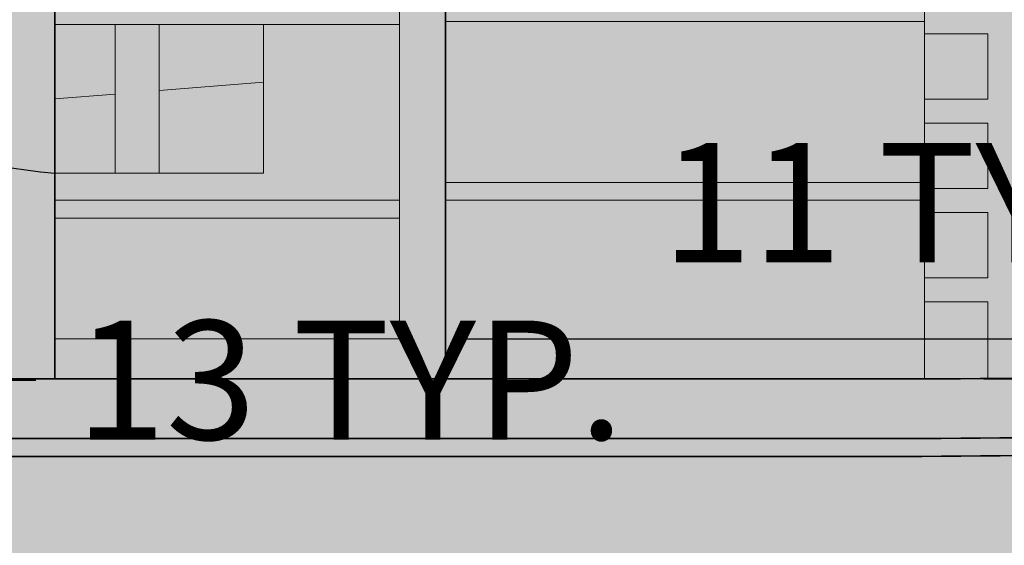
# Model space of a CAD drawing. Units: millimetres. Extents: x 130 to 1021, y 147 to 699.
# Tile 10 of 40: x 481 to 646, y 246 to 334. Entities that reach past the tile are written whole.
import ezdxf

# ---------------------------------------------------------------- set-up
doc = ezdxf.new("R2010")
doc.units = ezdxf.units.MM
doc.header["$MEASUREMENT"] = 0
for name, color, linetype, lineweight in [('A-ANNO-DIMS', 2, 'Continuous', 18), ('A-DOOR', 3, 'Continuous', 25), ('A-ELEV', 7, 'Continuous', 35), ('A-ELEV-PATT', 9, 'Continuous', 13), ('A-GLAZ', 4, 'Continuous', 18)]:
    doc.layers.add(name, color=color, linetype=linetype, lineweight=lineweight)
doc.styles.get("Standard").update_dxf_attribs({"font": 'arial.ttf'})
doc.dimstyles.get("Standard").update_dxf_attribs({"dimtxt": 20, "dimasz": 10, "dimexe": 10, "dimexo": 10, "dimgap": 5, "dimtad": 0, "dimtih": 1, "dimtoh": 1, "dimdec": 0, "dimzin": 0, "dimdsep": 46, "dimtxsty": 'Standard', "dimcen": 5, "dimadec": 0, "dimazin": 0, "dimtfac": 1, "dimtdec": 0, "dimtofl": 0, "dimtmove": 0, "dimatfit": 3, "dimfxl": 1, "dimtolj": 1, "dimtzin": 0, "dimarcsym": 0})

# ---------------------------------------------------------------- blocks, each defined once
blk = doc.blocks.new('*D6')
at = {"layer": 'A-ANNO-DIMS', "color": 0, "lineweight": -2, "transparency": 16777216}
for p, q in [((707.48, 311.89), (707.48, 313.54)), ((718.48, 311.89), (718.48, 313.54)), ((697.48, 303.54), (687.48, 303.54)), ((728.48, 303.54), (738.48, 303.54))]:
    blk.add_line(p, q, dxfattribs=at)
at = {"layer": 'A-ANNO-DIMS', "color": 0, "transparency": 16777216}
for points in [[(697.48, 305.21), (697.48, 301.87), (707.48, 303.54)], [(728.48, 305.21), (728.48, 301.87), (718.48, 303.54)]]:
    blk.add_solid(points, dxfattribs=at)
at = {"layer": 'Defpoints', "color": 0, "transparency": 16777216}
for p in [(707.48, 303.54), (707.48, 301.89), (718.48, 301.89)]:
    blk.add_point(p, dxfattribs=at)
at = {"layer": 'A-ANNO-DIMS', "color": 0, "transparency": 16777216, "insert": (634.74, 303.54), "char_height": 20, "attachment_point": 5}
blk.add_mtext('\\A1;11 TYP.', dxfattribs=at)
blk = doc.blocks.new('*D7')
at = {"layer": 'A-ANNO-DIMS', "color": 0, "lineweight": -2, "transparency": 16777216}
for p, q in [((399.37, 349.45), (413.37, 349.45)), ((423.37, 349.45), (433.37, 349.45)), ((389.37, 344.55), (389.37, 339.45)), ((423.37, 344.55), (423.37, 339.45))]:
    blk.add_line(p, q, dxfattribs=at)
at = {"layer": 'A-ANNO-DIMS', "color": 0, "transparency": 16777216}
for points in [[(399.37, 351.11), (399.37, 347.78), (389.37, 349.45)], [(413.37, 351.11), (413.37, 347.78), (423.37, 349.45)]]:
    blk.add_solid(points, dxfattribs=at)
at = {"layer": 'Defpoints', "color": 0, "transparency": 16777216}
for p in [(389.37, 354.55), (423.37, 354.55), (423.37, 349.45)]:
    blk.add_point(p, dxfattribs=at)
at = {"layer": 'A-ANNO-DIMS', "color": 0, "transparency": 16777216, "insert": (582.04, 349.45), "char_height": 20, "attachment_point": 5}
blk.add_mtext('\\A1;DOOR PANEL 34 TYP.', dxfattribs=at)
blk = doc.blocks.new('*D10')
at = {"layer": 'A-ANNO-DIMS', "color": 0, "lineweight": -2, "transparency": 16777216}
for p, q in [((440.89, 273.72), (430.89, 273.71)), ((473.57, 273.75), (483.57, 273.75)), ((450.9, 267.56), (450.9, 263.73)), ((463.58, 267.57), (463.58, 263.74))]:
    blk.add_line(p, q, dxfattribs=at)
at = {"layer": 'A-ANNO-DIMS', "color": 0, "transparency": 16777216}
for points in [[(440.89, 275.38), (440.89, 272.05), (450.89, 273.73)], [(473.57, 275.41), (473.58, 272.08), (463.57, 273.74)]]:
    blk.add_solid(points, dxfattribs=at)
at = {"layer": 'Defpoints', "color": 0, "transparency": 16777216}
for p in [(450.89, 277.56), (463.57, 277.57), (463.57, 273.74)]:
    blk.add_point(p, dxfattribs=at)
at = {"layer": 'A-ANNO-DIMS', "color": 0, "transparency": 16777216, "insert": (536.31, 273.75), "char_height": 20, "attachment_point": 5}
blk.add_mtext('\\A1;13 TYP.', dxfattribs=at)
blk = doc.blocks.new('*D11')
at = {"layer": 'A-ANNO-DIMS', "color": 0, "lineweight": -2, "transparency": 16777216}
for p, q in [((737.37, 648.7), (737.37, 149.74)), ((299.37, 566.95), (299.37, 149.74)), ((309.37, 159.74), (490.86, 159.74)), ((727.37, 159.74), (545.89, 159.74))]:
    blk.add_line(p, q, dxfattribs=at)
at = {"layer": 'A-ANNO-DIMS', "color": 0, "transparency": 16777216}
for points in [[(309.37, 161.41), (309.37, 158.07), (299.37, 159.74)], [(727.37, 161.41), (727.37, 158.07), (737.37, 159.74)]]:
    blk.add_solid(points, dxfattribs=at)
at = {"layer": 'Defpoints', "color": 0, "transparency": 16777216}
for p in [(737.37, 658.7), (299.37, 576.95), (737.37, 159.74)]:
    blk.add_point(p, dxfattribs=at)
at = {"layer": 'A-ANNO-DIMS', "color": 0, "transparency": 16777216, "insert": (518.37, 159.74), "char_height": 20, "attachment_point": 5}
blk.add_mtext('\\A1;438', dxfattribs=at)
blk = doc.blocks.new('*D12')
at = {"layer": 'A-ANNO-DIMS', "color": 0, "lineweight": -2, "transparency": 16777216}
for p, q in [((477.37, 661.95), (265.07, 661.95)), ((275.07, 651.95), (275.07, 438.2)), ((275.07, 194.04), (275.07, 407.78)), ((357.16, 184.04), (265.07, 184.04))]:
    blk.add_line(p, q, dxfattribs=at)
at = {"layer": 'A-ANNO-DIMS', "color": 0, "transparency": 16777216}
for points in [[(273.41, 651.95), (276.74, 651.95), (275.07, 661.95)], [(273.41, 194.04), (276.74, 194.04), (275.07, 184.04)]]:
    blk.add_solid(points, dxfattribs=at)
at = {"layer": 'Defpoints', "color": 0, "transparency": 16777216}
for p in [(275.07, 661.95), (487.37, 661.95), (367.16, 184.04)]:
    blk.add_point(p, dxfattribs=at)
at = {"layer": 'A-ANNO-DIMS', "color": 0, "transparency": 16777216, "insert": (275.07, 422.99), "char_height": 20, "attachment_point": 5}
blk.add_mtext('\\A1;477.9', dxfattribs=at)
blk = doc.blocks.new('*D23')
at = {"layer": 'A-ANNO-DIMS', "color": 0, "lineweight": -2, "transparency": 16777216}
for p, q in [((466.77, 403.95), (466.77, 696.25)), ((475.99, 209.04), (475.99, 696.25)), ((456.77, 686.25), (446.77, 686.25)), ((485.99, 686.25), (495.99, 686.25))]:
    blk.add_line(p, q, dxfattribs=at)
at = {"layer": 'A-ANNO-DIMS', "color": 0, "transparency": 16777216}
for points in [[(456.77, 687.91), (456.77, 684.58), (466.77, 686.25)], [(485.99, 687.91), (485.99, 684.58), (475.99, 686.25)]]:
    blk.add_solid(points, dxfattribs=at)
at = {"layer": 'Defpoints', "color": 0, "transparency": 16777216}
for p in [(475.99, 686.25), (466.77, 393.95), (475.99, 199.04)]:
    blk.add_point(p, dxfattribs=at)
at = {"layer": 'A-ANNO-DIMS', "color": 0, "transparency": 16777216, "insert": (534.63, 686.25), "char_height": 20, "attachment_point": 5}
blk.add_mtext('\\A1;9.222', dxfattribs=at)
blk = doc.blocks.new('*D24')
at = {"layer": 'A-ANNO-DIMS', "color": 0, "lineweight": -2, "transparency": 16777216}
for p, q in [((475.99, 209.04), (475.99, 696.25)), ((487.37, 671.95), (487.37, 696.25)), ((465.99, 686.25), (455.99, 686.25)), ((497.37, 686.25), (507.37, 686.25))]:
    blk.add_line(p, q, dxfattribs=at)
at = {"layer": 'A-ANNO-DIMS', "color": 0, "transparency": 16777216}
for points in [[(465.99, 687.91), (465.99, 684.58), (475.99, 686.25)], [(497.37, 687.91), (497.37, 684.58), (487.37, 686.25)]]:
    blk.add_solid(points, dxfattribs=at)
at = {"layer": 'Defpoints', "color": 0, "transparency": 16777216}
for p in [(487.37, 686.25), (487.37, 661.95), (475.99, 199.04)]:
    blk.add_point(p, dxfattribs=at)
at = {"layer": 'A-ANNO-DIMS', "color": 0, "transparency": 16777216, "insert": (553.02, 686.25), "char_height": 20, "attachment_point": 5}
blk.add_mtext('\\A1;11.385', dxfattribs=at)
blk = doc.blocks.new('*D49')
at = {"layer": 'A-ANNO-DIMS', "color": 0, "lineweight": -2, "transparency": 16777216}
for p, q in [((761.67, 283.95), (761.67, 293.95)), ((642.82, 273.95), (771.67, 273.95)), ((742.37, 213.95), (771.67, 213.95)), ((761.67, 203.95), (761.67, 193.95))]:
    blk.add_line(p, q, dxfattribs=at)
at = {"layer": 'A-ANNO-DIMS', "color": 0, "transparency": 16777216}
for points in [[(760.01, 283.95), (763.34, 283.95), (761.67, 273.95)], [(760.01, 203.95), (763.34, 203.95), (761.67, 213.95)]]:
    blk.add_solid(points, dxfattribs=at)
at = {"layer": 'Defpoints', "color": 0, "transparency": 16777216}
for p in [(632.82, 273.95), (761.67, 273.95), (732.37, 213.95)]:
    blk.add_point(p, dxfattribs=at)
at = {"layer": 'A-ANNO-DIMS', "color": 0, "transparency": 16777216, "insert": (761.67, 243.95), "char_height": 20, "attachment_point": 5}
blk.add_mtext('\\A1;60', dxfattribs=at)
blk = doc.blocks.new('*D50')
at = {"layer": 'A-ANNO-DIMS', "color": 0, "lineweight": -2, "transparency": 16777216}
for p, q in [((761.67, 290.66), (761.67, 300.66)), ((761.67, 300.66), (771.67, 300.66)), ((554.64, 280.66), (771.67, 280.66)), ((642.82, 273.95), (771.67, 273.95)), ((761.67, 263.95), (761.67, 253.95))]:
    blk.add_line(p, q, dxfattribs=at)
at = {"layer": 'A-ANNO-DIMS', "color": 0, "transparency": 16777216}
for points in [[(760.01, 290.66), (763.34, 290.66), (761.67, 280.66)], [(760.01, 263.95), (763.34, 263.95), (761.67, 273.95)]]:
    blk.add_solid(points, dxfattribs=at)
at = {"layer": 'Defpoints', "color": 0, "transparency": 16777216}
for p in [(544.64, 280.66), (761.67, 280.66), (632.82, 273.95)]:
    blk.add_point(p, dxfattribs=at)
at = {"layer": 'A-ANNO-DIMS', "color": 0, "transparency": 16777216, "insert": (810.55, 300.66), "char_height": 20, "attachment_point": 5}
blk.add_mtext('\\A1;6.715', dxfattribs=at)
blk = doc.blocks.new('*D51')
at = {"layer": 'A-ANNO-DIMS', "color": 0, "lineweight": -2, "transparency": 16777216}
for p, q in [((554.64, 386.26), (771.67, 386.26)), ((761.67, 376.26), (761.67, 348.67)), ((761.67, 290.66), (761.67, 318.25)), ((554.64, 280.66), (771.67, 280.66))]:
    blk.add_line(p, q, dxfattribs=at)
at = {"layer": 'A-ANNO-DIMS', "color": 0, "transparency": 16777216}
for points in [[(760.01, 376.26), (763.34, 376.26), (761.67, 386.26)], [(760.01, 290.66), (763.34, 290.66), (761.67, 280.66)]]:
    blk.add_solid(points, dxfattribs=at)
at = {"layer": 'Defpoints', "color": 0, "transparency": 16777216}
for p in [(544.64, 386.26), (761.67, 386.26), (544.64, 280.66)]:
    blk.add_point(p, dxfattribs=at)
at = {"layer": 'A-ANNO-DIMS', "color": 0, "transparency": 16777216, "insert": (761.67, 333.46), "char_height": 20, "attachment_point": 5}
blk.add_mtext('\\A1;105.6', dxfattribs=at)
blk = doc.blocks.new('*D61')
at = {"layer": 'A-ANNO-DIMS', "color": 0, "lineweight": -2, "transparency": 16777216}
for p, q in [((761.67, 390.89), (761.67, 400.89)), ((642.82, 380.89), (771.67, 380.89)), ((642.82, 365.89), (771.67, 365.89)), ((761.67, 355.89), (761.67, 345.89)), ((761.67, 345.89), (751.67, 345.89))]:
    blk.add_line(p, q, dxfattribs=at)
at = {"layer": 'A-ANNO-DIMS', "color": 0, "transparency": 16777216}
for points in [[(760.01, 390.89), (763.34, 390.89), (761.67, 380.89)], [(760.01, 355.89), (763.34, 355.89), (761.67, 365.89)]]:
    blk.add_solid(points, dxfattribs=at)
at = {"layer": 'Defpoints', "color": 0, "transparency": 16777216}
for p in [(632.82, 380.89), (632.82, 365.89), (761.67, 365.89)]:
    blk.add_point(p, dxfattribs=at)
at = {"layer": 'A-ANNO-DIMS', "color": 0, "transparency": 16777216, "insert": (733.22, 345.89), "char_height": 20, "attachment_point": 5}
blk.add_mtext('\\A1;15', dxfattribs=at)
blk = doc.blocks.new('*D64')
at = {"layer": 'A-ANNO-DIMS', "color": 0, "lineweight": -2, "transparency": 16777216}
for p, q in [((502.05, 450.93), (502.05, 460.93)), ((497.05, 455.93), (507.05, 455.93)), ((363.96, 263.06), (409.92, 327.25)), ((353.96, 263.06), (363.96, 263.06))]:
    blk.add_line(p, q, dxfattribs=at)
at = {"layer": 'A-ANNO-DIMS', "color": 0, "transparency": 16777216}
blk.add_solid([(408.57, 328.22), (411.28, 326.28), (415.74, 335.39)], dxfattribs=at)
at = {"layer": 'Defpoints', "color": 0, "transparency": 16777216}
for p in [(502.05, 455.93), (415.74, 335.39)]:
    blk.add_point(p, dxfattribs=at)
at = {"layer": 'A-ANNO-DIMS', "color": 0, "transparency": 16777216, "insert": (297.8, 263.06), "char_height": 20, "attachment_point": 5}
blk.add_mtext('\\A1;R148.25', dxfattribs=at)
blk = doc.blocks.new('*D65')
at = {"layer": 'A-ANNO-DIMS', "color": 0, "lineweight": -2, "transparency": 16777216}
for p, q in [((495.46, 509.13), (472.51, 423.11)), ((505.46, 509.13), (495.46, 509.13)), ((427.37, 248.98), (427.37, 258.98)), ((422.37, 253.98), (432.37, 253.98))]:
    blk.add_line(p, q, dxfattribs=at)
at = {"layer": 'A-ANNO-DIMS', "color": 0, "transparency": 16777216}
blk.add_solid([(470.9, 423.54), (474.12, 422.68), (469.93, 413.45)], dxfattribs=at)
at = {"layer": 'Defpoints', "color": 0, "transparency": 16777216}
for p in [(469.93, 413.45), (427.37, 253.98)]:
    blk.add_point(p, dxfattribs=at)
at = {"layer": 'A-ANNO-DIMS', "color": 0, "transparency": 16777216, "insert": (561.62, 509.13), "char_height": 20, "attachment_point": 5}
blk.add_mtext('\\A1;R165.05', dxfattribs=at)
blk = doc.blocks.new('*D67')
at = {"layer": 'A-ANNO-DIMS', "color": 0, "lineweight": -2, "transparency": 16777216}
for p, q in [((479.76, 492.43), (462.14, 412.22)), ((489.76, 492.43), (479.76, 492.43)), ((427.07, 247.5), (427.07, 257.5)), ((422.07, 252.5), (432.07, 252.5))]:
    blk.add_line(p, q, dxfattribs=at)
at = {"layer": 'A-ANNO-DIMS', "color": 0, "transparency": 16777216}
blk.add_solid([(460.52, 412.58), (463.77, 411.87), (460, 402.46)], dxfattribs=at)
at = {"layer": 'Defpoints', "color": 0, "transparency": 16777216}
for p in [(460, 402.46), (427.07, 252.5)]:
    blk.add_point(p, dxfattribs=at)
at = {"layer": 'A-ANNO-DIMS', "color": 0, "transparency": 16777216, "insert": (545.84, 492.43), "char_height": 20, "attachment_point": 5}
blk.add_mtext('\\A1;R153.53', dxfattribs=at)

msp = doc.modelspace()

# ---------------------------------------------------------------- hatches: boundary and pattern name
at = {"layer": 'A-ELEV-PATT'}
h = msp.add_hatch(color=256, dxfattribs=at)
h.dxf.hatch_style = 1
h.paths.add_polyline_path([(737.3738, 658.6988, 0.01359606), (632.4019, 661.9473), (607.3738, 661.9473), (487.3738, 661.9473), (487.3738, 649.9473), (607.3738, 649.9473), (632.3794, 649.9473, -0.01368411), (737.3738, 646.6784)])
h.paths.add_polyline_path([(732.3738, 643.9599, 0.01305286), (632.3738, 646.9473), (607.3738, 646.9473), (487.3738, 646.9473), (487.3738, 596.9473), (632.3738, 596.9473, -0.01305286), (732.3738, 593.9599)])
h.paths.add_polyline_path([(737.3738, 593.6732, 0.01370629), (632.3738, 596.9473), (487.3738, 596.9473), (487.3738, 586.9473), (632.355, 586.9473, -0.01378075), (737.3738, 583.6559)])
h.paths.add_polyline_path([(447.3738, 646.9473), (307.3738, 646.9473), (302.3738, 646.9473), (302.3738, 634.9473), (447.3738, 634.9473)])
h.paths.add_polyline_path([(447.3738, 631.9473), (307.3738, 631.9473), (307.3738, 586.9473), (447.3738, 586.9473)])
h.paths.add_polyline_path([(447.3738, 586.9473), (307.3738, 586.9473), (302.3738, 586.9473), (302.3738, 576.9473), (447.3738, 576.9473)])
h.paths.add_polyline_path([(447.3738, 573.9473), (367.3738, 573.9473), (367.3738, 539.9473), (447.3738, 539.9473)])
h.paths.add_polyline_path([(447.3738, 537.9473), (367.3738, 537.9473), (367.3738, 507.9473), (400.392, 507.4253, -0.00172798), (401.3281, 507.6451, -0.52200255), (425.6117, 511.0391, -0.03918489), (447.3738, 510.4359), (447.3738, 510.7883)])
h.paths.add_polyline_path([(394.7238, 505.9473), (367.3738, 505.9473), (367.3738, 476.9473, -0.0146512), (375.8501, 480.2159), (376.1506, 499.2266, -0.03554194)])
h.paths.add_polyline_path([(632.3738, 583.9473), (552.3738, 583.9473), (552.3738, 550.9473), (632.3738, 550.9473)])
h.paths.add_polyline_path([(632.3738, 548.9473), (552.3738, 548.9473), (552.3738, 515.9473), (632.3738, 515.9473)])
h.paths.add_polyline_path([(632.3738, 513.9473), (552.3738, 513.9473), (552.3738, 476.9473), (632.3738, 476.9473)])
h.paths.add_polyline_path([(737.3738, 473.6903, 0.01363261), (632.3926, 476.9473), (552.3738, 476.9473), (487.3738, 476.9473), (487.3738, 466.9473), (632.3738, 466.9473, -0.01370629), (737.3738, 463.6732)])
h.paths.add_polyline_path([(732.3738, 460.9552, 0.01307409), (632.3681, 463.9473), (487.3738, 463.9473), (487.3738, 407.735, -0.00322862), (489.3544, 406.9473), (632.3926, 406.9473, -0.01298259), (732.3738, 403.9755)])
h.paths.add_polyline_path([(487.3738, 463.9473, 0.20132998), (367.3738, 463.9473), (367.3738, 407.735, -0.18820307), (487.3738, 407.735)])
h.paths.add_polyline_path([(367.3738, 476.9473), (367.3738, 466.9473, -0.20133085), (487.3738, 466.9473), (487.3738, 476.9473, 0.20132998)])
h.paths.add_polyline_path([(367.3738, 463.9473), (307.3738, 463.9473), (307.3738, 401.9473), (357.9413, 401.9473), (367.3738, 407.735)])
h.paths.add_polyline_path([(367.3738, 476.9473), (302.3738, 476.9473), (302.3738, 466.9473), (367.3738, 466.9473)])
h.paths.add_polyline_path([(632.8184, 366.9453), (552.3738, 366.9453), (552.3738, 393.9473), (632.8184, 393.9473)])
h.paths.add_polyline_path([(632.8184, 357.2114), (632.8184, 363.9453), (552.3738, 363.9453), (552.3738, 357.2114), (552.3738, 336.9453), (632.8184, 336.9453)])
h.paths.add_polyline_path([(632.8184, 333.9453), (552.3738, 333.9453), (552.3738, 306.9453), (632.8184, 306.9453)])
h.paths.add_polyline_path([(632.8184, 303.9453), (552.3738, 303.9453), (552.3738, 273.9473), (632.355, 273.9473, 0.00006077), (632.8184, 273.9491)])
h.paths.add_polyline_path([(737.3738, 403.6903, 0.01363261), (632.3926, 406.9473), (489.3544, 406.9473, 0.19154808), (367.3738, 407.735), (367.3738, 396.9473, -0.20133085), (487.3738, 396.9473), (632.3738, 396.9473, -0.01370629), (737.3738, 393.6732)])
h.paths.add_polyline_path([(357.9413, 401.9473), (307.3738, 401.9473), (307.3738, 391.9473), (357.9413, 391.9473)])
h.paths.add_polyline_path([(357.9413, 357.2114), (357.9413, 388.9473), (307.3738, 388.9473), (307.3738, 357.2114), (307.3738, 273.9473), (357.9413, 273.9473)])
h.paths.add_polyline_path([(732.3738, 263.93, -0.0130317), (632.3794, 260.9473), (466.7667, 260.9473), (466.7667, 240.9473), (469.8406, 236.978), (469.8406, 221.978), (472.9145, 218.0087), (472.9145, 213.9473), (607.3738, 213.9473), (732.3738, 213.9473)])
h.paths.add_polyline_path([(732.3738, 290.889), (722.479, 290.889), (722.479, 301.889), (732.3738, 301.889), (732.3738, 305.889), (722.479, 305.889), (722.479, 316.889), (732.3738, 316.889), (732.3738, 320.889), (722.479, 320.889), (722.479, 331.889), (732.3738, 331.889), (732.3738, 335.889), (722.479, 335.889), (722.479, 346.889), (732.3738, 346.889), (732.3738, 350.889), (722.479, 350.889), (722.479, 361.889), (732.3738, 361.889), (732.3738, 365.889), (722.479, 365.889), (722.479, 376.889), (732.3738, 376.889), (732.3738, 380.889), (722.479, 380.889), (722.479, 391.4848, 0.00052326), (718.479, 391.6843), (718.479, 380.889), (707.479, 380.889), (707.479, 392.1896, 0.00052307), (703.479, 392.3576), (703.479, 380.889), (692.479, 380.889), (692.479, 392.7765, 0.00052292), (688.479, 392.9131), (688.479, 380.889), (677.479, 380.889), (677.479, 393.2456, 0.00052279), (673.479, 393.3508), (673.479, 380.889), (662.479, 380.889), (662.479, 393.597, 0.0005227), (658.479, 393.6709), (658.479, 380.889), (647.479, 380.889), (647.479, 393.8308, 0.00052264), (643.479, 393.8732), (643.479, 380.889), (632.8184, 380.889), (632.8184, 376.889), (643.479, 376.889), (643.479, 365.889), (632.8184, 365.889), (632.8184, 361.889), (643.479, 361.889), (643.479, 350.889), (632.8184, 350.889), (632.8184, 346.889), (643.479, 346.889), (643.479, 335.889), (632.8184, 335.889), (632.8184, 331.889), (643.479, 331.889), (643.479, 320.889), (632.8184, 320.889), (632.8184, 316.889), (643.479, 316.889), (643.479, 305.889), (632.8184, 305.889), (632.8184, 301.889), (643.479, 301.889), (643.479, 290.889), (632.8184, 290.889), (632.8184, 286.889), (643.479, 286.889), (643.479, 274.0217, 0.00052456), (647.479, 274.0643), (647.479, 286.889), (658.479, 286.889), (658.479, 274.2248, 0.00052462), (662.479, 274.2989), (662.479, 286.889), (673.479, 286.889), (673.479, 274.546, 0.00052471), (677.479, 274.6516), (677.479, 286.889), (688.479, 286.889), (688.479, 274.9853, 0.00052484), (692.479, 275.1224), (692.479, 286.889), (703.479, 286.889), (703.479, 275.5429, 0.000525), (707.479, 275.7115), (707.479, 286.889), (718.479, 286.889), (718.479, 276.2187, 0.00052519), (722.479, 276.4189), (722.479, 286.889), (732.3738, 286.889)])
h.paths.add_polyline_path([(718.479, 290.889), (707.479, 290.889), (707.479, 301.889), (718.479, 301.889)], flags=16)
h.paths.add_polyline_path([(703.479, 290.889), (692.479, 290.889), (692.479, 301.889), (703.479, 301.889)], flags=16)
h.paths.add_polyline_path([(718.479, 305.889), (707.479, 305.889), (707.479, 316.889), (718.479, 316.889)], flags=16)
h.paths.add_polyline_path([(703.479, 305.889), (692.479, 305.889), (692.479, 316.889), (703.479, 316.889)], flags=16)
h.paths.add_polyline_path([(688.479, 290.889), (677.479, 290.889), (677.479, 301.889), (688.479, 301.889)], flags=16)
h.paths.add_polyline_path([(718.479, 320.889), (707.479, 320.889), (707.479, 331.889), (718.479, 331.889)], flags=16)
h.paths.add_polyline_path([(688.479, 305.889), (677.479, 305.889), (677.479, 316.889), (688.479, 316.889)], flags=16)
h.paths.add_polyline_path([(703.479, 320.889), (692.479, 320.889), (692.479, 331.889), (703.479, 331.889)], flags=16)
h.paths.add_polyline_path([(688.479, 320.889), (677.479, 320.889), (677.479, 331.889), (688.479, 331.889)], flags=16)
h.paths.add_polyline_path([(673.479, 290.889), (662.479, 290.889), (662.479, 301.889), (673.479, 301.889)], flags=16)
h.paths.add_polyline_path([(718.479, 335.889), (707.479, 335.889), (707.479, 346.889), (718.479, 346.889)], flags=16)
h.paths.add_polyline_path([(673.479, 305.889), (662.479, 305.889), (662.479, 316.889), (673.479, 316.889)], flags=16)
h.paths.add_polyline_path([(703.479, 335.889), (692.479, 335.889), (692.479, 346.889), (703.479, 346.889)], flags=16)
h.paths.add_polyline_path([(673.479, 320.889), (662.479, 320.889), (662.479, 331.889), (673.479, 331.889)], flags=16)
h.paths.add_polyline_path([(688.479, 335.889), (677.479, 335.889), (677.479, 346.889), (688.479, 346.889)], flags=16)
h.paths.add_polyline_path([(658.479, 290.889), (647.479, 290.889), (647.479, 301.889), (658.479, 301.889)], flags=16)
h.paths.add_polyline_path([(718.479, 350.889), (707.479, 350.889), (707.479, 361.889), (718.479, 361.889)], flags=16)
h.paths.add_polyline_path([(658.479, 305.889), (647.479, 305.889), (647.479, 316.889), (658.479, 316.889)], flags=16)
h.paths.add_polyline_path([(703.479, 350.889), (692.479, 350.889), (692.479, 361.889), (703.479, 361.889)], flags=16)
h.paths.add_polyline_path([(673.479, 335.889), (662.479, 335.889), (662.479, 346.889), (673.479, 346.889)], flags=16)
h.paths.add_polyline_path([(658.479, 320.889), (647.479, 320.889), (647.479, 331.889), (658.479, 331.889)], flags=16)
h.paths.add_polyline_path([(688.479, 350.889), (677.479, 350.889), (677.479, 361.889), (688.479, 361.889)], flags=16)
h.paths.add_polyline_path([(718.479, 365.889), (707.479, 365.889), (707.479, 376.889), (718.479, 376.889)], flags=16)
h.paths.add_polyline_path([(658.479, 335.889), (647.479, 335.889), (647.479, 346.889), (658.479, 346.889)], flags=16)
h.paths.add_polyline_path([(673.479, 350.889), (662.479, 350.889), (662.479, 361.889), (673.479, 361.889)], flags=16)
h.paths.add_polyline_path([(703.479, 365.889), (692.479, 365.889), (692.479, 376.889), (703.479, 376.889)], flags=16)
h.paths.add_polyline_path([(688.479, 365.889), (677.479, 365.889), (677.479, 376.889), (688.479, 376.889)], flags=16)
h.paths.add_polyline_path([(658.479, 350.889), (647.479, 350.889), (647.479, 361.889), (658.479, 361.889)], flags=16)
h.paths.add_polyline_path([(673.479, 365.889), (662.479, 365.889), (662.479, 376.889), (673.479, 376.889)], flags=16)
h.paths.add_polyline_path([(658.479, 365.889), (647.479, 365.889), (647.479, 376.889), (658.479, 376.889)], flags=16)
h.paths.add_polyline_path([(732.3738, 503.9786), (722.3392, 503.9786), (722.3392, 514.9786), (732.3738, 514.9786), (732.3738, 518.9786), (722.3392, 518.9786), (722.3392, 529.9786), (732.3738, 529.9786), (732.3738, 533.9786), (722.3392, 533.9786), (722.3392, 544.9786), (732.3738, 544.9786), (732.3738, 546.9473), (732.3738, 548.9786), (722.3392, 548.9786), (722.3392, 559.9786), (732.3738, 559.9786), (732.3738, 563.9786), (722.3392, 563.9786), (722.3392, 574.9786), (732.3738, 574.9786), (732.3738, 578.9786), (722.3392, 578.9786), (722.3392, 581.4789, 0.00052601), (718.3392, 581.6791), (718.3392, 578.9786), (707.3392, 578.9786), (707.3392, 582.1863, 0.00052582), (703.3392, 582.355), (703.3392, 578.9786), (692.3392, 578.9786), (692.3392, 582.7752, 0.00052566), (688.3392, 582.9123), (688.3392, 578.9786), (677.3392, 578.9786), (677.3392, 583.2457, 0.00052554), (673.3392, 583.3512), (673.3392, 578.9786), (662.3392, 578.9786), (662.3392, 583.5978, 0.00052545), (658.3392, 583.6718), (658.3392, 578.9786), (647.3392, 578.9786), (647.3392, 583.8317, 0.00052539), (643.3392, 583.8741), (643.3392, 578.9786), (632.3738, 578.9786), (632.3738, 574.9786), (643.3392, 574.9786), (643.3392, 563.9786), (632.3738, 563.9786), (632.3738, 559.9786), (643.3392, 559.9786), (643.3392, 548.9786), (632.3738, 548.9786), (632.3738, 544.9786), (643.3392, 544.9786), (643.3392, 533.9786), (632.3738, 533.9786), (632.3738, 529.9786), (643.3392, 529.9786), (643.3392, 518.9786), (632.3738, 518.9786), (632.3738, 515.9473), (632.3738, 514.9786), (643.3392, 514.9786), (643.3392, 503.9786), (632.3738, 503.9786), (632.3738, 499.9786), (643.3392, 499.9786), (643.3392, 488.9786), (632.3738, 488.9786), (632.3738, 484.9786), (643.3392, 484.9786), (643.3392, 476.8751, -0.00051911), (647.3392, 476.8332), (647.3392, 484.9786), (658.3392, 484.9786), (658.3392, 476.6752, -0.00051917), (662.3392, 476.6022), (662.3392, 484.9786), (673.3392, 484.9786), (673.3392, 476.3585, -0.00051926), (677.3392, 476.2543), (677.3392, 484.9786), (688.3392, 484.9786), (688.3392, 475.9248, -0.00051938), (692.3392, 475.7894), (692.3392, 484.9786), (703.3392, 484.9786), (703.3392, 475.3741, -0.00051953), (707.3392, 475.2075), (707.3392, 484.9786), (718.3392, 484.9786), (718.3392, 474.7064, -0.00051972), (722.3392, 474.5086), (722.3392, 484.9786), (732.3738, 484.9786), (732.3738, 488.9786), (722.3392, 488.9786), (722.3392, 499.9786), (732.3738, 499.9786)])
h.paths.add_polyline_path([(718.3392, 503.9786), (707.3392, 503.9786), (707.3392, 514.9786), (718.3392, 514.9786)], flags=16)
h.paths.add_polyline_path([(718.3392, 499.9786), (718.3392, 488.9786), (707.3392, 488.9786), (707.3392, 499.9786)], flags=16)
h.paths.add_polyline_path([(718.3392, 518.9786), (707.3392, 518.9786), (707.3392, 529.9786), (718.3392, 529.9786)], flags=16)
h.paths.add_polyline_path([(703.3392, 503.9786), (692.3392, 503.9786), (692.3392, 514.9786), (703.3392, 514.9786)], flags=16)
h.paths.add_polyline_path([(703.3392, 499.9786), (703.3392, 488.9786), (692.3392, 488.9786), (692.3392, 499.9786)], flags=16)
h.paths.add_polyline_path([(703.3392, 518.9786), (692.3392, 518.9786), (692.3392, 529.9786), (703.3392, 529.9786)], flags=16)
h.paths.add_polyline_path([(718.3392, 533.9786), (707.3392, 533.9786), (707.3392, 544.9786), (718.3392, 544.9786)], flags=16)
h.paths.add_polyline_path([(688.3392, 503.9786), (677.3392, 503.9786), (677.3392, 514.9786), (688.3392, 514.9786)], flags=16)
h.paths.add_polyline_path([(688.3392, 499.9786), (688.3392, 488.9786), (677.3392, 488.9786), (677.3392, 499.9786)], flags=16)
h.paths.add_polyline_path([(703.3392, 533.9786), (692.3392, 533.9786), (692.3392, 544.9786), (703.3392, 544.9786)], flags=16)
h.paths.add_polyline_path([(688.3392, 518.9786), (677.3392, 518.9786), (677.3392, 529.9786), (688.3392, 529.9786)], flags=16)
h.paths.add_polyline_path([(688.3392, 533.9786), (677.3392, 533.9786), (677.3392, 544.9786), (688.3392, 544.9786)], flags=16)
h.paths.add_polyline_path([(718.3392, 548.9786), (707.3392, 548.9786), (707.3392, 559.9786), (718.3392, 559.9786)], flags=16)
h.paths.add_polyline_path([(673.3392, 503.9786), (662.3392, 503.9786), (662.3392, 514.9786), (673.3392, 514.9786)], flags=16)
h.paths.add_polyline_path([(673.3392, 499.9786), (673.3392, 488.9786), (662.3392, 488.9786), (662.3392, 499.9786)], flags=16)
h.paths.add_polyline_path([(703.3392, 548.9786), (692.3392, 548.9786), (692.3392, 559.9786), (703.3392, 559.9786)], flags=16)
h.paths.add_polyline_path([(673.3392, 518.9786), (662.3392, 518.9786), (662.3392, 529.9786), (673.3392, 529.9786)], flags=16)
h.paths.add_polyline_path([(688.3392, 548.9786), (677.3392, 548.9786), (677.3392, 559.9786), (688.3392, 559.9786)], flags=16)
h.paths.add_polyline_path([(673.3392, 533.9786), (662.3392, 533.9786), (662.3392, 544.9786), (673.3392, 544.9786)], flags=16)
h.paths.add_polyline_path([(718.3392, 563.9786), (707.3392, 563.9786), (707.3392, 574.9786), (718.3392, 574.9786)], flags=16)
h.paths.add_polyline_path([(658.3392, 503.9786), (647.3392, 503.9786), (647.3392, 514.9786), (658.3392, 514.9786)], flags=16)
h.paths.add_polyline_path([(658.3392, 499.9786), (658.3392, 488.9786), (647.3392, 488.9786), (647.3392, 499.9786)], flags=16)
h.paths.add_polyline_path([(703.3392, 563.9786), (692.3392, 563.9786), (692.3392, 574.9786), (703.3392, 574.9786)], flags=16)
h.paths.add_polyline_path([(658.3392, 518.9786), (647.3392, 518.9786), (647.3392, 529.9786), (658.3392, 529.9786)], flags=16)
h.paths.add_polyline_path([(673.3392, 548.9786), (662.3392, 548.9786), (662.3392, 559.9786), (673.3392, 559.9786)], flags=16)
h.paths.add_polyline_path([(688.3392, 563.9786), (677.3392, 563.9786), (677.3392, 574.9786), (688.3392, 574.9786)], flags=16)
h.paths.add_polyline_path([(658.3392, 533.9786), (647.3392, 533.9786), (647.3392, 544.9786), (658.3392, 544.9786)], flags=16)
h.paths.add_polyline_path([(673.3392, 563.9786), (662.3392, 563.9786), (662.3392, 574.9786), (673.3392, 574.9786)], flags=16)
h.paths.add_polyline_path([(658.3392, 548.9786), (647.3392, 548.9786), (647.3392, 559.9786), (658.3392, 559.9786)], flags=16)
h.paths.add_polyline_path([(658.3392, 563.9786), (647.3392, 563.9786), (647.3392, 574.9786), (658.3392, 574.9786)], flags=16)
h = msp.add_hatch(color=256, dxfattribs=at)
h.dxf.hatch_style = 1
h.paths.add_polyline_path([(447.3738, 576.9473), (302.3738, 576.9473), (302.3738, 573.9473), (447.3738, 573.9473)])
h.paths.add_polyline_path([(487.3738, 583.9473), (487.3738, 586.9473), (447.3738, 576.9473), (447.3738, 573.9473)])
h.paths.add_polyline_path([(632.355, 586.9473), (487.3738, 586.9473), (487.3738, 583.9473), (632.3738, 583.9473), (632.3738, 583.9472, -0.01380003), (737.3738, 580.6507), (737.3738, 583.6559, 0.01378075)])
h.paths.add_polyline_path([(367.3738, 466.9473), (302.3738, 466.9473), (302.3738, 463.9473), (367.3738, 463.9473)])
h.paths.add_polyline_path([(487.3738, 463.9473), (487.3738, 466.9473, 0.20133085), (367.3738, 466.9473), (367.3738, 463.9473, -0.20132998)])
h.paths.add_polyline_path([(632.3738, 466.9473), (487.3738, 466.9473), (487.3738, 463.9473), (632.3681, 463.9473, -0.01372855), (737.3738, 460.6681), (737.3738, 463.6732, 0.01370629)])
h.paths.add_polyline_path([(632.3738, 396.9473), (487.3738, 396.9473, 0.20133085), (367.3738, 396.9473), (367.3738, 393.9473, -0.20237172), (486.7667, 393.9473), (632.3681, 393.9473, -0.01372855), (737.3738, 390.6681), (737.3738, 393.6732, 0.01370629)])
h.paths.add_polyline_path([(357.9413, 391.9473), (307.3738, 391.9473), (307.3738, 388.9473), (357.9413, 388.9473)])
h.paths.add_polyline_path([(367.3738, 393.9473), (367.3738, 396.9473), (357.9413, 391.924), (357.9413, 388.9473), (358.058, 388.9473)])
h.paths.add_polyline_path([(737.3738, 264.2162), (737.3738, 267.2214, -0.01370629), (632.3738, 263.9473), (463.7667, 263.9473), (466.7667, 260.9473), (632.3794, 260.9473, 0.01368411)])
h.paths.add_polyline_path([(463.7667, 263.9473), (447.3738, 263.9473), (450.3738, 260.9473), (466.7667, 260.9473)])
h.paths.add_polyline_path([(447.3738, 263.9473), (432.3738, 263.9473), (432.3738, 260.9473), (450.3738, 260.9473)])
h.paths.add_polyline_path([(382.3738, 263.9473), (357.9413, 263.9473), (357.9413, 260.9473), (382.3738, 260.9473)])
h.paths.add_polyline_path([(357.9413, 263.9473), (307.3738, 263.9473), (307.3738, 260.9473), (357.9413, 260.9473)])
h = msp.add_hatch(color=256, dxfattribs=at)
h.paths.add_polyline_path([(327.3738, 569.884), (327.3738, 573.9473), (307.3738, 573.9473), (307.3738, 476.9473), (327.3738, 476.9473), (327.3738, 480.95)])
h.paths.add_polyline_path([(486.7667, 386.2639), (486.7667, 393.9473), (466.7667, 393.9473), (466.7667, 357.2114), (466.7667, 311.9335, 0.03427026), (486.7667, 308.4637)])
h.paths.add_polyline_path([(486.7667, 308.4637, -0.03427026), (466.7667, 311.9335), (466.7667, 273.9473), (486.7667, 273.9473)])
h.paths.add_polyline_path([(389.3738, 351.5473), (396.7693, 351.5473, -0.00702703), (393.8774, 354.5473), (389.3738, 354.5473), (389.3738, 359.5775, -0.01903024), (382.3738, 368.424), (382.3738, 249.5473), (432.3738, 249.5473), (432.3738, 325.067, -0.00576734), (429.3738, 326.709), (429.3738, 257.5473), (426.3738, 257.5473), (426.3738, 328.4428, -0.00592542), (423.3738, 330.272), (423.3738, 315.7473), (389.3738, 315.7473), (389.3738, 332.1473), (420.4552, 332.1473, -0.00895099), (416.0768, 335.1473), (389.3738, 335.1473)])
h.paths.add_polyline_path([(389.3738, 312.7473), (423.3738, 312.7473), (423.3738, 296.3473), (389.3738, 296.3473)], flags=16)
h.paths.add_polyline_path([(389.3738, 293.3473), (423.3738, 293.3473), (423.3738, 276.9473), (389.3738, 276.9473)], flags=16)
h.paths.add_polyline_path([(389.3738, 273.9473), (423.3738, 273.9473), (423.3738, 257.5473), (389.3738, 257.5473)], flags=16)
h.paths.add_polyline_path([(432.3738, 378.9473), (382.3738, 378.9473), (382.3738, 368.424, 0.01903024), (389.3738, 359.5775), (389.3738, 370.9473), (423.3738, 370.9473), (423.3738, 354.5473), (393.8774, 354.5473, 0.00702703), (396.7693, 351.5473), (423.3738, 351.5473), (423.3738, 335.1473), (416.0768, 335.1473, 0.00895099), (420.4552, 332.1473), (423.3738, 332.1473), (423.3738, 330.272, 0.00592542), (426.3738, 328.4428), (426.3738, 370.9473), (429.3738, 370.9473), (429.3738, 326.709, 0.00576734), (432.3738, 325.067)])
h.paths.add_polyline_path([(466.7667, 357.2114), (466.7667, 393.9473), (447.3738, 393.9473), (447.3738, 357.2114), (447.3738, 318.1243, 0.0063261), (450.8779, 316.785), (450.8779, 331.5915), (463.5608, 331.5915), (463.5608, 312.7571, 0.00558197), (466.7667, 311.9335)])
h.paths.add_polyline_path([(450.8779, 334.5915), (450.8779, 360.0915), (463.5608, 360.0915), (463.5608, 334.5915)], flags=16)
h.paths.add_polyline_path([(450.8779, 363.0915), (450.8779, 388.6449), (463.5608, 388.6449), (463.5608, 363.0915)], flags=16)
h.paths.add_polyline_path([(466.7667, 311.9335, -0.00558197), (463.5608, 312.7571), (463.5608, 306.0915), (450.8779, 306.0915), (450.8779, 316.785, -0.0063261), (447.3738, 318.1243), (447.3738, 273.9473), (466.7667, 273.9473)])
h.paths.add_polyline_path([(450.8779, 303.0915), (463.5608, 303.0915), (463.5608, 277.5915), (450.8779, 277.5915)], flags=16)
h.paths.add_polyline_path([(552.3738, 357.2114), (552.3738, 393.9473), (486.7667, 393.9473), (486.7667, 386.2639), (544.6354, 386.2639), (544.6354, 280.6619), (486.7667, 280.6619), (486.7667, 273.9473), (552.3738, 273.9473)])
h.paths.add_polyline_path([(487.3738, 583.9473), (472.3738, 580.1973), (472.3738, 507.0765), (472.3738, 505.4251, -0.00564525), (475.3738, 504.4942), (475.3738, 506.3543), (475.3738, 511.9473), (484.3738, 511.9473), (484.3738, 503.8134), (484.3738, 501.2439, -0.00583574), (487.3738, 500.0015)])
h.paths.add_polyline_path([(484.3738, 578.0434), (484.3738, 548.9473), (475.3738, 548.9473), (475.3738, 575.7934)], flags=16)
h.paths.add_polyline_path([(484.3738, 546.9473), (484.3738, 513.9473), (475.3738, 513.9473), (475.3738, 518.7148), (475.3738, 546.9473)], flags=16)
h = msp.add_hatch(color=256, dxfattribs=at)
h.dxf.hatch_style = 1
h.paths.add_polyline_path([(447.3738, 537.9473), (447.3738, 539.9473), (367.3738, 539.9473), (367.3738, 537.9473)])
h.paths.add_polyline_path([(394.7238, 505.9473, -0.0105284), (400.392, 507.4253), (367.3738, 507.9473), (367.3738, 505.9473)])
h.paths.add_polyline_path([(547.7773, 546.9473), (547.7773, 548.9473), (502.3738, 548.9473), (502.3738, 546.9473)])
h.paths.add_polyline_path([(632.3738, 548.9473), (632.3738, 550.9473), (552.3738, 550.9473), (552.3738, 548.9473)])
h.paths.add_polyline_path([(632.3738, 513.9473), (632.3738, 515.9473), (552.3738, 515.9473), (552.3738, 513.9473)])
h.paths.add_polyline_path([(544.6354, 360.9453), (544.6354, 363.9453), (486.7667, 363.9454), (486.7667, 360.9454)])
h.paths.add_polyline_path([(632.8184, 363.9453), (632.8184, 366.9453), (552.3738, 366.9453), (552.3738, 363.9453)])
h.paths.add_polyline_path([(632.8184, 333.9453), (632.8184, 336.9453), (552.3738, 336.9453), (552.3738, 333.9453)])
h.paths.add_polyline_path([(552.3738, 306.9453), (552.3738, 303.9453), (632.8184, 303.9453), (632.8184, 306.9453)])
h = msp.add_hatch(color=256, dxfattribs=at)
h.set_gradient(color1=(0, 153, 204), color2=(102, 204, 127))
h.paths.add_polyline_path([(643.479, 286.889), (632.8184, 286.889), (632.8184, 273.9491, 0.00139799), (643.479, 274.0217)])
h.paths.add_polyline_path([(647.479, 274.0643, 0.00144261), (658.479, 274.2248), (658.479, 286.889), (647.479, 286.889)])
h.paths.add_polyline_path([(662.479, 274.2989, 0.00144282), (673.479, 274.546), (673.479, 286.889), (662.479, 286.889)])
h.paths.add_polyline_path([(677.479, 274.6516, 0.00144312), (688.479, 274.9853), (688.479, 286.889), (677.479, 286.889)])
h.paths.add_polyline_path([(703.479, 275.5429), (703.479, 286.889), (692.479, 286.889), (692.479, 275.1224, 0.00144351)])
h.paths.add_polyline_path([(707.479, 275.7115, 0.00144399), (718.479, 276.2187), (718.479, 286.889), (707.479, 286.889)])
h.paths.add_polyline_path([(722.479, 276.4189, 0.0012994), (732.3738, 276.9505), (732.3738, 286.889), (722.479, 286.889)])
h.paths.add_polyline_path([(722.479, 290.889), (732.3738, 290.889), (732.3738, 301.889), (722.479, 301.889)])
h.paths.add_polyline_path([(718.479, 301.889), (707.479, 301.889), (707.479, 290.889), (718.479, 290.889)])
h.paths.add_polyline_path([(703.479, 301.889), (692.479, 301.889), (692.479, 290.889), (703.479, 290.889)])
h.paths.add_polyline_path([(677.479, 290.889), (688.479, 290.889), (688.479, 301.889), (677.479, 301.889)])
h.paths.add_polyline_path([(673.479, 301.889), (662.479, 301.889), (662.479, 290.889), (673.479, 290.889)])
h.paths.add_polyline_path([(658.479, 301.889), (647.479, 301.889), (647.479, 290.889), (658.479, 290.889)])
h.paths.add_polyline_path([(643.479, 301.889), (632.8184, 301.889), (632.8184, 290.889), (643.479, 290.889)])
h.paths.add_polyline_path([(643.479, 316.889), (632.8184, 316.889), (632.8184, 305.889), (643.479, 305.889)])
h.paths.add_polyline_path([(647.479, 305.889), (658.479, 305.889), (658.479, 316.889), (647.479, 316.889)])
h.paths.add_polyline_path([(662.479, 305.889), (673.479, 305.889), (673.479, 316.889), (662.479, 316.889)])
h.paths.add_polyline_path([(688.479, 316.889), (677.479, 316.889), (677.479, 305.889), (688.479, 305.889)])
h.paths.add_polyline_path([(692.479, 305.889), (703.479, 305.889), (703.479, 316.889), (692.479, 316.889)])
h.paths.add_polyline_path([(707.479, 305.889), (718.479, 305.889), (718.479, 316.889), (707.479, 316.889)])
h.paths.add_polyline_path([(722.479, 305.889), (732.3738, 305.889), (732.3738, 316.889), (722.479, 316.889)])
h.paths.add_polyline_path([(732.3738, 331.889), (722.479, 331.889), (722.479, 320.889), (732.3738, 320.889)])
h.paths.add_polyline_path([(718.479, 331.889), (707.479, 331.889), (707.479, 320.889), (718.479, 320.889)])
h.paths.add_polyline_path([(703.479, 331.889), (692.479, 331.889), (692.479, 320.889), (703.479, 320.889)])
h.paths.add_polyline_path([(688.479, 331.889), (677.479, 331.889), (677.479, 320.889), (688.479, 320.889)])
h.paths.add_polyline_path([(673.479, 331.889), (662.479, 331.889), (662.479, 320.889), (673.479, 320.889)])
h.paths.add_polyline_path([(647.479, 320.889), (658.479, 320.889), (658.479, 331.889), (647.479, 331.889)])
h.paths.add_polyline_path([(643.479, 320.889), (643.479, 331.889), (632.8184, 331.889), (632.8184, 320.889)])
h.paths.add_polyline_path([(632.8184, 335.889), (643.479, 335.889), (643.479, 346.889), (632.8184, 346.889)])
h.paths.add_polyline_path([(647.479, 335.889), (658.479, 335.889), (658.479, 346.889), (647.479, 346.889)])
h.paths.add_polyline_path([(673.479, 346.889), (662.479, 346.889), (662.479, 335.889), (673.479, 335.889)])
h.paths.add_polyline_path([(677.479, 335.889), (688.479, 335.889), (688.479, 346.889), (677.479, 346.889)])
h.paths.add_polyline_path([(703.479, 346.889), (692.479, 346.889), (692.479, 335.889), (703.479, 335.889)])
h.paths.add_polyline_path([(707.479, 335.889), (718.479, 335.889), (718.479, 346.889), (707.479, 346.889)])
h.paths.add_polyline_path([(722.479, 335.889), (732.3738, 335.889), (732.3738, 346.889), (722.479, 346.889)])
h.paths.add_polyline_path([(722.479, 361.889), (722.479, 350.889), (732.3738, 350.889), (732.3738, 357.2114), (732.3738, 361.889)])
h.paths.add_polyline_path([(707.479, 350.889), (718.479, 350.889), (718.479, 361.889), (707.479, 361.889)])
h.paths.add_polyline_path([(703.479, 361.889), (692.479, 361.889), (692.479, 350.889), (703.479, 350.889)])
h.paths.add_polyline_path([(688.479, 361.889), (677.479, 361.889), (677.479, 350.889), (688.479, 350.889)])
h.paths.add_polyline_path([(662.479, 350.889), (673.479, 350.889), (673.479, 361.889), (662.479, 361.889)])
h.paths.add_polyline_path([(658.479, 350.889), (658.479, 361.889), (647.479, 361.889), (647.479, 350.889)])
h.paths.add_polyline_path([(643.479, 350.889), (643.479, 361.889), (632.8184, 361.889), (632.8184, 357.2114), (632.8184, 350.889)])
h.paths.add_polyline_path([(643.479, 376.889), (632.8184, 376.889), (632.8184, 365.889), (643.479, 365.889)])
h.paths.add_polyline_path([(658.479, 365.889), (658.479, 376.889), (647.479, 376.889), (647.479, 365.889)])
h.paths.add_polyline_path([(662.479, 365.889), (673.479, 365.889), (673.479, 376.889), (662.479, 376.889)])
h.paths.add_polyline_path([(688.479, 365.889), (688.479, 376.889), (677.479, 376.889), (677.479, 365.889)])
h.paths.add_polyline_path([(703.479, 365.889), (703.479, 376.889), (692.479, 376.889), (692.479, 365.889)])
h.paths.add_polyline_path([(718.479, 376.889), (707.479, 376.889), (707.479, 365.889), (718.479, 365.889)])
h.paths.add_polyline_path([(732.3738, 365.889), (732.3738, 376.889), (722.479, 376.889), (722.479, 365.889)])
h.paths.add_polyline_path([(722.479, 380.889), (732.3738, 380.889), (732.3738, 390.9552, 0.00129463), (722.479, 391.4848)])
h.paths.add_polyline_path([(718.479, 391.6843, 0.0014387), (707.479, 392.1896), (707.479, 380.889), (718.479, 380.889)])
h.paths.add_polyline_path([(703.479, 392.3576, 0.00143822), (692.479, 392.7765), (692.479, 380.889), (703.479, 380.889)])
h.paths.add_polyline_path([(677.479, 380.889), (688.479, 380.889), (688.479, 392.9131, 0.00143784), (677.479, 393.2456)])
h.paths.add_polyline_path([(662.479, 380.889), (673.479, 380.889), (673.479, 393.3508, 0.00143754), (662.479, 393.597)])
h.paths.add_polyline_path([(647.479, 380.889), (658.479, 380.889), (658.479, 393.6709, 0.00143733), (647.479, 393.8308)])
h.paths.add_polyline_path([(632.8184, 393.9456), (632.8184, 380.889), (643.479, 380.889), (643.479, 393.8732, 0.00139288)])
for points in [[(486.7667, 336.9454), (486.7667, 333.4629), (544.6354, 333.4629), (544.6354, 336.9453)], [(486.7667, 303.9454), (486.7667, 300.9454), (544.6354, 300.9453), (544.6354, 303.9453)]]:
    msp.add_hatch(color=256, dxfattribs=at).paths.add_polyline_path(points)
h = msp.add_hatch(color=256, dxfattribs=at)
h.set_gradient(color1=(0, 255, 0), color2=(0, 0, 0), name='CURVED')
h.paths.add_polyline_path([(521.8017, 323.7412), (504.2842, 322.3522), (504.2842, 308.4637), (521.8017, 308.4637)])
h.paths.add_polyline_path([(521.8017, 333.4629), (504.2842, 333.4629), (504.2842, 322.3522), (521.8017, 323.7412)])
h.paths.add_polyline_path([(496.8642, 333.4629), (486.7667, 333.4629), (486.7667, 320.9633), (496.8642, 321.7639)])
h.paths.add_polyline_path([(496.8642, 321.7639), (486.7667, 320.9633), (486.7667, 308.4637), (496.8642, 308.4637)])
h = msp.add_hatch(color=256, dxfattribs=at)
h.paths.add_polyline_path([(544.6354, 333.4629), (521.8017, 333.4629), (521.8017, 308.4637), (486.7667, 308.4637), (486.7667, 303.9454), (544.6354, 303.9453)])
h.paths.add_polyline_path([(504.2842, 333.4629), (496.8642, 333.4629), (496.8642, 308.4637), (504.2842, 308.4637)], flags=17)
h.paths.add_polyline_path([(544.6354, 300.9453), (486.7667, 300.9454), (486.7667, 280.6619), (544.6354, 280.6619)])
h = msp.add_hatch(color=256, dxfattribs=at)
h.dxf.hatch_style = 1
h.paths.add_polyline_path([(463.7667, 273.9473), (463.7667, 263.9473), (632.3738, 263.9473, 0.01370629), (737.3738, 267.2214), (737.3738, 277.2387, -0.01378075), (632.355, 273.9473)])

# ---------------------------------------------------------------- linework, layer by layer
at = {"layer": 'A-DOOR'}
msp.add_arc((502.0489, 455.9263), 148.2524, 204.712441, 264.083334, dxfattribs=at)
at = {"layer": 'A-ELEV'}
for p, q in [((486.7667, 357.2114), (486.7667, 273.9473)), ((552.3738, 357.2114), (552.3738, 273.9473)), ((432.3738, 273.9473), (632.3738, 273.9473)), ((432.3738, 263.9473), (632.3738, 263.9473)), ((432.3738, 260.9473), (632.3738, 260.9473))]:
    msp.add_line(p, q, dxfattribs=at)
for radius, end in [(1906.4697, 273.3741542), (1916.4697, 273.3565279), (1919.4697, 273.3512758)]:
    msp.add_arc((625.1665, 2180.4035), radius, 270.215474, end, dxfattribs=at)
at = {"layer": 'A-GLAZ'}
for p, q in [((632.8184, 273.9473), (632.8184, 357.2114)), ((544.6354, 333.4629), (486.7667, 333.4629)), ((552.3738, 333.9453), (632.8184, 333.9453)), ((632.8184, 331.889), (643.479, 331.889)), ((643.479, 320.889), (643.479, 331.889)), ((521.8017, 323.7412), (504.2842, 322.3522)), ((496.8642, 321.7639), (486.7667, 320.9633)), ((632.8184, 320.889), (643.479, 320.889)), ((632.8184, 316.889), (643.479, 316.889)), ((643.479, 305.889), (643.479, 316.889)), ((552.3738, 306.9453), (632.8184, 306.9453)), ((632.8184, 305.889), (643.479, 305.889)), ((486.7667, 303.9454), (544.6354, 303.9453)), ((552.3738, 303.9453), (632.8184, 303.9453)), ((632.8184, 301.889), (643.479, 301.889)), ((643.479, 290.889), (643.479, 301.889)), ((486.7667, 300.9454), (544.6354, 300.9453)), ((632.8184, 290.889), (643.479, 290.889)), ((632.8184, 286.889), (643.479, 286.889)), ((643.479, 273.9473), (643.479, 286.889))]:
    msp.add_line(p, q, dxfattribs=at)
msp.add_lwpolyline([(544.6354, 386.2639), (486.7667, 386.2639), (486.7667, 280.6619), (544.6354, 280.6619)], close=True, dxfattribs=at)
for points in [[(521.8017, 333.4629), (521.8017, 308.4637), (486.7667, 308.4637)], [(496.8642, 308.4637), (496.8642, 333.4629)], [(496.8642, 333.4629), (504.2842, 333.4629)], [(504.2842, 333.4629), (504.2842, 308.4637)]]:
    msp.add_lwpolyline(points, dxfattribs=at)

# ---------------------------------------------------------------- dimensions: what is measured, and where the dimension line sits
at = {"layer": 'A-ANNO-DIMS'}
for base, p1, p2, override, picture, middle in [((475.9885, 686.2473), (466.7667, 393.9473), (475.9885, 199.0395), {"dimdec": 3, "dimlfac": 1, "dimrnd": 0, "dimzin": 0, "dimdsep": 46, "dimlunit": 2}, '*D23', (534.631, 686.2473)), ((487.3738, 686.2473), (475.9885, 199.0395), (487.3738, 661.9473), {"dimdec": 3, "dimlfac": 1, "dimrnd": 0, "dimzin": 0, "dimdsep": 46, "dimlunit": 2}, '*D24', (553.0218, 686.2473)), ((737.3738, 159.7395), (299.3738, 576.9473), (737.3738, 658.6988), {"dimdec": 0, "dimlfac": 1, "dimrnd": 0, "dimzin": 0, "dimdsep": 46, "dimlunit": 2}, '*D11', (518.3738, 159.7395))]:
    dim = msp.add_linear_dim(base=base, p1=p1, p2=p2, dimstyle='Standard', override=override, dxfattribs=at)
    dim.commit()
    dim.dimension.update_dxf_attribs({"geometry": picture, "text_midpoint": middle})
for base, p1, p2, override, picture, middle in [((275.0738, 661.9473), (367.163, 184.0395), (487.3738, 661.9473), {"dimdec": 1, "dimlfac": 1, "dimrnd": 0, "dimzin": 0, "dimdsep": 46, "dimlunit": 2}, '*D12', (275.0738, 422.9934)), ((761.6738, 365.889), (632.8184, 380.889), (632.8184, 365.889), {"dimdec": 0, "dimlfac": 1, "dimrnd": 0, "dimzin": 0, "dimdsep": 46, "dimlunit": 2}, '*D61', (733.2154, 345.889)), ((761.6738, 386.2639), (544.6354, 280.6619), (544.6354, 386.2639), {"dimdec": 1, "dimlfac": 1, "dimrnd": 0, "dimzin": 0, "dimdsep": 46, "dimlunit": 2}, '*D51', (761.6738, 333.4629)), ((761.6738, 280.6619), (632.8184, 273.9473), (544.6354, 280.6619), {"dimdec": 3, "dimlfac": 1, "dimrnd": 0, "dimzin": 0, "dimdsep": 46, "dimlunit": 2}, '*D50', (810.5483, 300.6619)), ((761.6738, 273.9473), (732.3738, 213.9473), (632.8184, 273.9473), {"dimdec": 0, "dimlfac": 1, "dimrnd": 0, "dimzin": 0, "dimdsep": 46, "dimlunit": 2}, '*D49', (761.6738, 243.9473))]:
    dim = msp.add_linear_dim(base=base, p1=p1, p2=p2, angle=90, dimstyle='Standard', override=override, dxfattribs=at)
    dim.commit()
    dim.dimension.update_dxf_attribs({"geometry": picture, "text_midpoint": middle})
for center, mpoint, picture, middle in [((427.3738, 253.9788), (469.9297, 413.4465), '*D65', (561.6228, 509.1272)), ((427.0702, 252.4956), (459.999, 402.4554), '*D67', (545.8408, 492.4313)), ((502.0489, 455.9263), (415.7433, 335.3854), '*D64', (297.8003, 263.0608))]:
    dim = msp.add_radius_dim(center=center, mpoint=mpoint, dimstyle='Standard', override={"dimdec": 2, "dimlfac": 1, "dimrnd": 0, "dimzin": 0, "dimdsep": 46, "dimlunit": 2}, dxfattribs=at)
    dim.commit()
    dim.dimension.update_dxf_attribs({"geometry": picture, "text_midpoint": middle, "dimtype": 164})
dim = msp.add_linear_dim(base=(423.3738, 349.4473), p1=(389.3738, 354.5473), p2=(423.3738, 354.5473), text='DOOR PANEL <> TYP.', dimstyle='Standard', override={"dimdec": 0, "dimrnd": 0, "dimzin": 0, "dimlunit": 2}, dxfattribs=at)
dim.commit()
dim.dimension.update_dxf_attribs({"geometry": '*D7', "text_midpoint": (582.0368, 349.4473)})
for base, p1, p2, angle, picture, middle in [((707.479, 303.539), (718.479, 301.889), (707.479, 301.889), 180, '*D6', (634.7437, 303.539)), ((463.5746, 273.7371), (450.8885, 277.5595), (463.5714, 277.5701), 0.047753, '*D10', (536.3099, 273.7537))]:
    dim = msp.add_linear_dim(base=base, p1=p1, p2=p2, angle=angle, text='<> TYP.', dimstyle='Standard', override={"dimdec": 0, "dimrnd": 0, "dimzin": 0, "dimlunit": 2}, dxfattribs=at)
    dim.commit()
    dim.dimension.update_dxf_attribs({"geometry": picture, "text_midpoint": middle})

doc.saveas('drawing.dxf')
